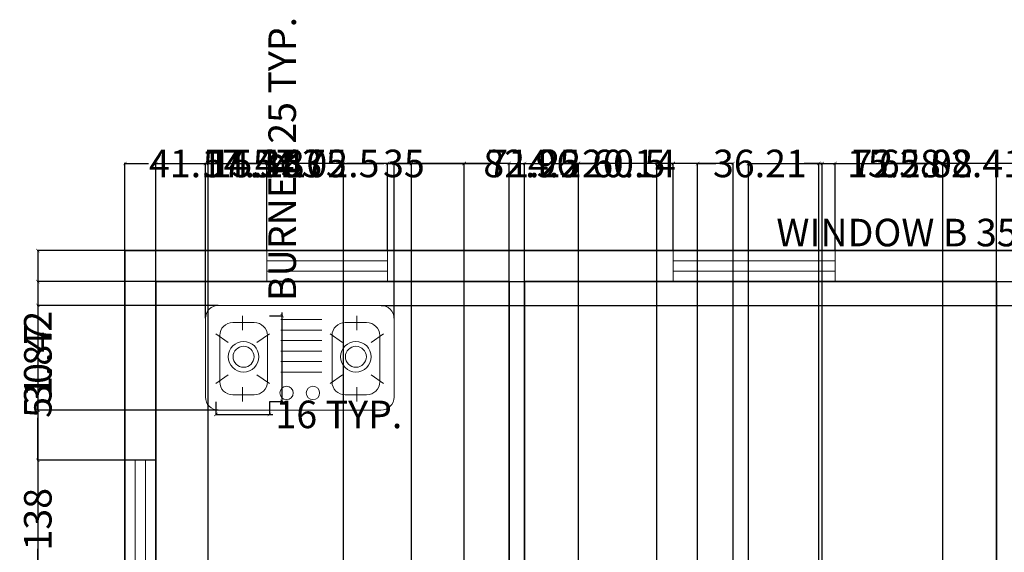
# Model space of a CAD drawing. Units: inches. Extents: x 878 to 1443, y 634 to 1188.
# Tile 3 of 5: x 878 to 1164, y 1033 to 1188. Entities that reach past the tile are written whole.
import ezdxf

# ---------------------------------------------------------------- set-up
doc = ezdxf.new("R2010")
doc.units = ezdxf.units.IN
doc.header["$MEASUREMENT"] = 0
doc.layers.add('A-ANNO-DIMS', color=2, linetype='Continuous', lineweight=18)
doc.layers.add('A-WALL', color=7, linetype='Continuous', lineweight=35)
doc.layers.add('A-GLAZ', color=152, linetype='Continuous', lineweight=18, true_color=0x2776bb)
doc.layers.add('Furniture', color=7, linetype='Continuous', lineweight=15, true_color=0xffffff)
doc.styles.get("Standard").update_dxf_attribs({"font": 'arial.ttf'})
doc.dimstyles.get("Standard").update_dxf_attribs({"dimtxt": 8, "dimasz": 1, "dimexe": 0.18, "dimexo": 0.0625, "dimgap": 0.09, "dimtad": 0, "dimdec": 4, "dimzin": 0, "dimdsep": 46, "dimlunit": 3, "dimtxsty": 'Standard', "dimblk": 'ARCHTICK', "dimcen": 0.09, "dimclrd": 6, "dimclre": 5, "dimclrt": 140, "dimadec": 0, "dimazin": 0, "dimtfac": 1, "dimtdec": 4, "dimtofl": 0, "dimtmove": 0, "dimatfit": 3, "dimfxl": 1, "dimtolj": 1, "dimtzin": 0, "dimarcsym": 0})

# ---------------------------------------------------------------- blocks, each defined once
blk = doc.blocks.new('WIN-47IN')
for p, q in [((9, 47), (0, 47)), ((0, 47), (0, 0)), ((3, 0), (3, 47)), ((6, 0), (6, 47)), ((9, 0), (9, 47)), ((0, 0), (9, 0))]:
    blk.add_line(p, q)
blk = doc.blocks.new('COOKTOP-BURNER')
for p, q in [((11.15, 22.96), (4.91, 22.96)), ((7.76, 24.89), (7.76, 20.74)), ((0, 19.64), (3.6, 17.15)), ((1.11, 19.15), (1.11, 5.74)), ((15.51, 19.64), (11.91, 17.15)), ((14.96, 5.74), (14.96, 19.15)), ((0, 5.25), (3.6, 7.74)), ((15.51, 5.25), (11.91, 7.74)), ((7.76, 0), (7.76, 4.15)), ((4.91, 1.94), (11.15, 1.94))]:
    blk.add_line(p, q)
for radius in [4.43, 3.05]:
    blk.add_circle((8.03, 13), radius)
for centre, start, end in [((4.91, 19.15), 90, 180), ((11.15, 19.15), 0, 90), ((4.91, 5.74), 180, 270), ((11.15, 5.74), 270, 0)]:
    blk.add_arc(centre, 3.8, start, end)
blk = doc.blocks.new('WIN-35IN')
for p, q in [((0, 35), (0, 0)), ((9, 35), (0, 35)), ((3, 0), (3, 35)), ((6, 0), (6, 35)), ((9, 0), (9, 35)), ((0, 0), (9, 0))]:
    blk.add_line(p, q)
blk = doc.blocks.new('_ArchTick')
at = {"color": 0, "linetype": 'ByBlock', "const_width": 0.15}
blk.add_lwpolyline([(-0.5, -0.5), (0.5, 0.5)], dxfattribs=at)
blk = doc.blocks.new('*D11')
at = {"layer": 'A-ANNO-DIMS', "color": 6, "lineweight": -2, "transparency": 16777216}
for p, q in [((1197.44, 1125.72), (1196.44, 1125.72)), ((1232.44, 1125.72), (1197.44, 1125.72))]:
    blk.add_line(p, q, dxfattribs=at)
at = {"layer": 'A-ANNO-DIMS', "color": 5, "lineweight": -2, "transparency": 16777216}
for p, q in [((1197.44, 1120.53), (1197.44, 1125.9)), ((1232.44, 1120.53), (1232.44, 1125.9))]:
    blk.add_line(p, q, dxfattribs=at)
at = {"layer": 'Defpoints', "color": 0, "lineweight": -2, "transparency": 16777216}
for p in [(1197.44, 1125.72), (1197.44, 1120.47), (1232.44, 1120.47)]:
    blk.add_point(p, dxfattribs=at)
at = {"layer": 'A-ANNO-DIMS', "color": 6, "lineweight": -2, "transparency": 16777216}
for p, rotation in [((1197.44, 1125.72), 179.9999999999992), ((1232.44, 1125.72), 359.9999999999992)]:
    blk.add_blockref('_ArchTick', p, dxfattribs=dict(at, rotation=rotation))
at = {"layer": 'A-ANNO-DIMS', "color": 140, "transparency": 16777216, "insert": (1145.37, 1125.72), "char_height": 8, "attachment_point": 5}
blk.add_mtext('\\A1;WINDOW B 35 TYP.', dxfattribs=at)
blk = doc.blocks.new('*D19')
at = {"layer": 'A-ANNO-DIMS', "color": 5, "lineweight": -2, "transparency": 16777216}
for p, q in [((950.87, 1101.54), (954.72, 1101.54)), ((950.87, 1076.65), (954.72, 1076.65))]:
    blk.add_line(p, q, dxfattribs=at)
at = {"layer": 'A-ANNO-DIMS', "color": 6, "lineweight": -2, "transparency": 16777216}
for p, q in [((954.54, 1101.54), (954.54, 1102.54)), ((954.54, 1076.65), (954.54, 1101.54))]:
    blk.add_line(p, q, dxfattribs=at)
at = {"layer": 'Defpoints', "color": 0, "lineweight": -2, "transparency": 16777216}
for p in [(950.81, 1101.54), (954.54, 1101.54), (950.81, 1076.65)]:
    blk.add_point(p, dxfattribs=at)
at = {"layer": 'A-ANNO-DIMS', "color": 6, "lineweight": -2, "transparency": 16777216}
for p, rotation in [((954.54, 1101.54), 90), ((954.54, 1076.65), 270)]:
    blk.add_blockref('_ArchTick', p, dxfattribs=dict(at, rotation=rotation))
at = {"layer": 'A-ANNO-DIMS', "color": 140, "transparency": 16777216, "insert": (954.54, 1147.08), "char_height": 8, "attachment_point": 5, "rotation": 90}
blk.add_mtext('\\A1;BURNER 25 TYP.', dxfattribs=at)
blk = doc.blocks.new('*D20')
at = {"layer": 'A-ANNO-DIMS', "color": 5, "lineweight": -2, "transparency": 16777216}
for p, q in [((935.3, 1076.59), (935.3, 1072.74)), ((950.81, 1076.59), (950.81, 1072.74))]:
    blk.add_line(p, q, dxfattribs=at)
at = {"layer": 'A-ANNO-DIMS', "color": 6, "lineweight": -2, "transparency": 16777216}
for p, q in [((935.3, 1072.92), (950.81, 1072.92)), ((950.81, 1072.92), (951.81, 1072.92))]:
    blk.add_line(p, q, dxfattribs=at)
at = {"layer": 'Defpoints', "color": 0, "lineweight": -2, "transparency": 16777216}
for p in [(935.3, 1076.65), (950.81, 1076.65), (950.81, 1072.92)]:
    blk.add_point(p, dxfattribs=at)
at = {"layer": 'A-ANNO-DIMS', "color": 6, "lineweight": -2, "transparency": 16777216, "rotation": 180}
blk.add_blockref('_ArchTick', (935.3, 1072.92), dxfattribs=at)
at = {"layer": 'A-ANNO-DIMS', "color": 6, "lineweight": -2, "transparency": 16777216}
blk.add_blockref('_ArchTick', (950.81, 1072.92), dxfattribs=at)
at = {"layer": 'A-ANNO-DIMS', "color": 140, "transparency": 16777216, "insert": (970.99, 1072.92), "char_height": 8, "attachment_point": 5}
blk.add_mtext('\\A1;16 TYP.', dxfattribs=at)
blk = doc.blocks.new('*D22')
at = {"layer": 'A-ANNO-DIMS', "color": 5, "lineweight": -2, "transparency": 16777216}
for p, q in [((908.84, 1120.47), (883.41, 1120.47)), ((908.84, 664.47), (883.41, 664.47))]:
    blk.add_line(p, q, dxfattribs=at)
at = {"layer": 'A-ANNO-DIMS', "color": 6, "lineweight": -2, "transparency": 16777216}
for p, q in [((883.59, 1120.47), (883.59, 901.56)), ((883.59, 664.47), (883.59, 883.38))]:
    blk.add_line(p, q, dxfattribs=at)
at = {"layer": 'Defpoints', "color": 0, "lineweight": -2, "transparency": 16777216}
for p in [(883.59, 1120.47), (908.9, 1120.47), (908.9, 664.47)]:
    blk.add_point(p, dxfattribs=at)
at = {"layer": 'A-ANNO-DIMS', "color": 6, "lineweight": -2, "transparency": 16777216}
for p, rotation in [((883.59, 1120.47), 90), ((883.59, 664.47), 270)]:
    blk.add_blockref('_ArchTick', p, dxfattribs=dict(at, rotation=rotation))
at = {"layer": 'A-ANNO-DIMS', "color": 140, "transparency": 16777216, "insert": (883.59, 892.47), "char_height": 8, "attachment_point": 5, "rotation": 90}
blk.add_mtext('\\A1;456', dxfattribs=at)
blk = doc.blocks.new('*D24')
at = {"layer": 'A-ANNO-DIMS', "color": 5, "lineweight": -2, "transparency": 16777216}
for p, q in [((908.9, 1120.53), (908.9, 1145.96)), ((950.07, 1120.53), (950.07, 1145.96))]:
    blk.add_line(p, q, dxfattribs=at)
at = {"layer": 'A-ANNO-DIMS', "color": 6, "lineweight": -2, "transparency": 16777216}
for p, q in [((908.9, 1145.78), (915.74, 1145.78)), ((950.07, 1145.78), (943.23, 1145.78))]:
    blk.add_line(p, q, dxfattribs=at)
at = {"layer": 'Defpoints', "color": 0, "lineweight": -2, "transparency": 16777216}
for p in [(950.07, 1145.78), (908.9, 1120.47), (950.07, 1120.47)]:
    blk.add_point(p, dxfattribs=at)
at = {"layer": 'A-ANNO-DIMS', "color": 6, "lineweight": -2, "transparency": 16777216, "rotation": 180}
blk.add_blockref('_ArchTick', (908.9, 1145.78), dxfattribs=at)
at = {"layer": 'A-ANNO-DIMS', "color": 6, "lineweight": -2, "transparency": 16777216}
blk.add_blockref('_ArchTick', (950.07, 1145.78), dxfattribs=at)
at = {"layer": 'A-ANNO-DIMS', "color": 140, "transparency": 16777216, "insert": (929.49, 1145.78), "char_height": 8, "attachment_point": 5}
blk.add_mtext('\\A1;41.17', dxfattribs=at)
blk = doc.blocks.new('*D25')
at = {"layer": 'A-ANNO-DIMS', "color": 5, "lineweight": -2, "transparency": 16777216}
for p, q in [((985.07, 1120.53), (985.07, 1145.96)), ((1068.03, 1120.53), (1068.03, 1145.96))]:
    blk.add_line(p, q, dxfattribs=at)
at = {"layer": 'A-ANNO-DIMS', "color": 6, "lineweight": -2, "transparency": 16777216}
for p, q in [((985.07, 1145.78), (1012.96, 1145.78)), ((1068.03, 1145.78), (1040.14, 1145.78))]:
    blk.add_line(p, q, dxfattribs=at)
at = {"layer": 'Defpoints', "color": 0, "lineweight": -2, "transparency": 16777216}
for p in [(1068.03, 1145.78), (985.07, 1120.47), (1068.03, 1120.47)]:
    blk.add_point(p, dxfattribs=at)
at = {"layer": 'A-ANNO-DIMS', "color": 6, "lineweight": -2, "transparency": 16777216, "rotation": 180}
blk.add_blockref('_ArchTick', (985.07, 1145.78), dxfattribs=at)
at = {"layer": 'A-ANNO-DIMS', "color": 6, "lineweight": -2, "transparency": 16777216}
blk.add_blockref('_ArchTick', (1068.03, 1145.78), dxfattribs=at)
at = {"layer": 'A-ANNO-DIMS', "color": 140, "transparency": 16777216, "insert": (1026.55, 1145.78), "char_height": 8, "attachment_point": 5}
blk.add_mtext('\\A1;82.96', dxfattribs=at)
blk = doc.blocks.new('*D26')
at = {"layer": 'A-ANNO-DIMS', "color": 5, "lineweight": -2, "transparency": 16777216}
for p, q in [((1115.03, 1120.53), (1115.03, 1145.96)), ((1197.44, 1120.53), (1197.44, 1145.96))]:
    blk.add_line(p, q, dxfattribs=at)
at = {"layer": 'A-ANNO-DIMS', "color": 6, "lineweight": -2, "transparency": 16777216}
for p, q in [((1115.03, 1145.78), (1143.42, 1145.78)), ((1197.44, 1145.78), (1169.06, 1145.78))]:
    blk.add_line(p, q, dxfattribs=at)
at = {"layer": 'Defpoints', "color": 0, "lineweight": -2, "transparency": 16777216}
for p in [(1197.44, 1145.78), (1115.03, 1120.47), (1197.44, 1120.47)]:
    blk.add_point(p, dxfattribs=at)
at = {"layer": 'A-ANNO-DIMS', "color": 6, "lineweight": -2, "transparency": 16777216, "rotation": 180}
blk.add_blockref('_ArchTick', (1115.03, 1145.78), dxfattribs=at)
at = {"layer": 'A-ANNO-DIMS', "color": 6, "lineweight": -2, "transparency": 16777216}
blk.add_blockref('_ArchTick', (1197.44, 1145.78), dxfattribs=at)
at = {"layer": 'A-ANNO-DIMS', "color": 140, "transparency": 16777216, "insert": (1156.24, 1145.78), "char_height": 8, "attachment_point": 5}
blk.add_mtext('\\A1;82.41', dxfattribs=at)
blk = doc.blocks.new('*D29')
at = {"layer": 'A-ANNO-DIMS', "color": 5, "lineweight": -2, "transparency": 16777216}
for p, q in [((917.84, 1111.47), (883.41, 1111.47)), ((917.84, 1059.6), (883.41, 1059.6))]:
    blk.add_line(p, q, dxfattribs=at)
at = {"layer": 'A-ANNO-DIMS', "color": 6, "lineweight": -2, "transparency": 16777216}
for p, q in [((883.59, 1111.47), (883.59, 1099.12)), ((883.59, 1059.6), (883.59, 1071.95))]:
    blk.add_line(p, q, dxfattribs=at)
at = {"layer": 'Defpoints', "color": 0, "lineweight": -2, "transparency": 16777216}
for p in [(917.9, 1111.47), (883.59, 1059.6), (917.9, 1059.6)]:
    blk.add_point(p, dxfattribs=at)
at = {"layer": 'A-ANNO-DIMS', "color": 6, "lineweight": -2, "transparency": 16777216}
for p, rotation in [((883.59, 1111.47), 90), ((883.59, 1059.6), 270)]:
    blk.add_blockref('_ArchTick', p, dxfattribs=dict(at, rotation=rotation))
at = {"layer": 'A-ANNO-DIMS', "color": 140, "transparency": 16777216, "insert": (883.59, 1085.53), "char_height": 8, "attachment_point": 5, "rotation": 90}
blk.add_mtext('\\A1;51.87', dxfattribs=at)
blk = doc.blocks.new('*D33')
at = {"layer": 'A-ANNO-DIMS', "color": 5, "lineweight": -2, "transparency": 16777216}
for p, q in [((917.9, 760.53), (917.9, 1145.96)), ((1020.4, 760.53), (1020.4, 1145.96))]:
    blk.add_line(p, q, dxfattribs=at)
at = {"layer": 'A-ANNO-DIMS', "color": 6, "lineweight": -2, "transparency": 16777216}
for p, q in [((917.9, 1145.78), (955.91, 1145.78)), ((1020.4, 1145.78), (982.39, 1145.78))]:
    blk.add_line(p, q, dxfattribs=at)
at = {"layer": 'Defpoints', "color": 0, "lineweight": -2, "transparency": 16777216}
for p in [(1020.4, 1145.78), (917.9, 760.47), (1020.4, 760.47)]:
    blk.add_point(p, dxfattribs=at)
at = {"layer": 'A-ANNO-DIMS', "color": 6, "lineweight": -2, "transparency": 16777216, "rotation": 180}
blk.add_blockref('_ArchTick', (917.9, 1145.78), dxfattribs=at)
at = {"layer": 'A-ANNO-DIMS', "color": 6, "lineweight": -2, "transparency": 16777216}
blk.add_blockref('_ArchTick', (1020.4, 1145.78), dxfattribs=at)
at = {"layer": 'A-ANNO-DIMS', "color": 140, "transparency": 16777216, "insert": (969.15, 1145.78), "char_height": 8, "attachment_point": 5}
blk.add_mtext('\\A1;102.5', dxfattribs=at)
blk = doc.blocks.new('*D34')
at = {"layer": 'A-ANNO-DIMS', "color": 5, "lineweight": -2, "transparency": 16777216}
for p, q in [((1024.9, 1111.41), (1024.9, 638.98)), ((1161.9, 1111.41), (1161.9, 638.98))]:
    blk.add_line(p, q, dxfattribs=at)
at = {"layer": 'A-ANNO-DIMS', "color": 6, "lineweight": -2, "transparency": 16777216}
for p, q in [((1024.9, 639.16), (1084.85, 639.16)), ((1161.9, 639.16), (1101.95, 639.16))]:
    blk.add_line(p, q, dxfattribs=at)
at = {"layer": 'Defpoints', "color": 0, "lineweight": -2, "transparency": 16777216}
for p in [(1024.9, 1111.47), (1161.9, 1111.47), (1161.9, 639.16)]:
    blk.add_point(p, dxfattribs=at)
at = {"layer": 'A-ANNO-DIMS', "color": 6, "lineweight": -2, "transparency": 16777216, "rotation": 180}
blk.add_blockref('_ArchTick', (1024.9, 639.16), dxfattribs=at)
at = {"layer": 'A-ANNO-DIMS', "color": 6, "lineweight": -2, "transparency": 16777216}
blk.add_blockref('_ArchTick', (1161.9, 639.16), dxfattribs=at)
at = {"layer": 'A-ANNO-DIMS', "color": 140, "transparency": 16777216, "insert": (1093.4, 639.16), "char_height": 8, "attachment_point": 5}
blk.add_mtext('\\A1;137', dxfattribs=at)
blk = doc.blocks.new('*D36')
at = {"layer": 'A-ANNO-DIMS', "color": 5, "lineweight": -2, "transparency": 16777216}
for p, q in [((1020.34, 1111.47), (883.41, 1111.47)), ((1020.34, 973.47), (883.41, 973.47))]:
    blk.add_line(p, q, dxfattribs=at)
at = {"layer": 'A-ANNO-DIMS', "color": 6, "lineweight": -2, "transparency": 16777216}
for p, q in [((883.59, 1111.47), (883.59, 1051.03)), ((883.59, 973.47), (883.59, 1033.91))]:
    blk.add_line(p, q, dxfattribs=at)
at = {"layer": 'Defpoints', "color": 0, "lineweight": -2, "transparency": 16777216}
for p in [(1020.4, 1111.47), (883.59, 973.47), (1020.4, 973.47)]:
    blk.add_point(p, dxfattribs=at)
at = {"layer": 'A-ANNO-DIMS', "color": 6, "lineweight": -2, "transparency": 16777216}
for p, rotation in [((883.59, 1111.47), 90), ((883.59, 973.47), 270)]:
    blk.add_blockref('_ArchTick', p, dxfattribs=dict(at, rotation=rotation))
at = {"layer": 'A-ANNO-DIMS', "color": 140, "transparency": 16777216, "insert": (883.59, 1042.47), "char_height": 8, "attachment_point": 5, "rotation": 90}
blk.add_mtext('\\A1;138', dxfattribs=at)
blk = doc.blocks.new('*D39')
at = {"layer": 'A-ANNO-DIMS', "color": 5, "lineweight": -2, "transparency": 16777216}
for p, q in [((1024.9, 880.53), (1024.9, 1145.96)), ((1085.4, 880.53), (1085.4, 1145.96))]:
    blk.add_line(p, q, dxfattribs=at)
at = {"layer": 'A-ANNO-DIMS', "color": 6, "lineweight": -2, "transparency": 16777216}
for p, q in [((1024.9, 1145.78), (1044.62, 1145.78)), ((1085.4, 1145.78), (1065.68, 1145.78))]:
    blk.add_line(p, q, dxfattribs=at)
at = {"layer": 'Defpoints', "color": 0, "lineweight": -2, "transparency": 16777216}
for p in [(1085.4, 1145.78), (1024.9, 880.47), (1085.4, 880.47)]:
    blk.add_point(p, dxfattribs=at)
at = {"layer": 'A-ANNO-DIMS', "color": 6, "lineweight": -2, "transparency": 16777216, "rotation": 180}
blk.add_blockref('_ArchTick', (1024.9, 1145.78), dxfattribs=at)
at = {"layer": 'A-ANNO-DIMS', "color": 6, "lineweight": -2, "transparency": 16777216}
blk.add_blockref('_ArchTick', (1085.4, 1145.78), dxfattribs=at)
at = {"layer": 'A-ANNO-DIMS', "color": 140, "transparency": 16777216, "insert": (1055.15, 1145.78), "char_height": 8, "attachment_point": 5}
blk.add_mtext('\\A1;60.5', dxfattribs=at)
blk = doc.blocks.new('*D40')
at = {"layer": 'A-ANNO-DIMS', "color": 5, "lineweight": -2, "transparency": 16777216}
for p, q in [((1089.9, 880.53), (1089.9, 1145.96)), ((1161.9, 880.53), (1161.9, 1145.96))]:
    blk.add_line(p, q, dxfattribs=at)
at = {"layer": 'A-ANNO-DIMS', "color": 6, "lineweight": -2, "transparency": 16777216}
for p, q in [((1089.9, 1145.78), (1120.15, 1145.78)), ((1161.9, 1145.78), (1131.64, 1145.78))]:
    blk.add_line(p, q, dxfattribs=at)
at = {"layer": 'Defpoints', "color": 0, "lineweight": -2, "transparency": 16777216}
for p in [(1161.9, 1145.78), (1089.9, 880.47), (1161.9, 880.47)]:
    blk.add_point(p, dxfattribs=at)
at = {"layer": 'A-ANNO-DIMS', "color": 6, "lineweight": -2, "transparency": 16777216, "rotation": 180}
blk.add_blockref('_ArchTick', (1089.9, 1145.78), dxfattribs=at)
at = {"layer": 'A-ANNO-DIMS', "color": 6, "lineweight": -2, "transparency": 16777216}
blk.add_blockref('_ArchTick', (1161.9, 1145.78), dxfattribs=at)
at = {"layer": 'A-ANNO-DIMS', "color": 140, "transparency": 16777216, "insert": (1125.9, 1145.78), "char_height": 8, "attachment_point": 5}
blk.add_mtext('\\A1;72', dxfattribs=at)
blk = doc.blocks.new('*D44')
at = {"layer": 'A-ANNO-DIMS', "color": 5, "lineweight": -2, "transparency": 16777216}
for p, q in [((917.9, 751.53), (917.9, 1145.96)), ((933.09, 751.53), (933.09, 1145.96))]:
    blk.add_line(p, q, dxfattribs=at)
at = {"layer": 'A-ANNO-DIMS', "color": 6, "lineweight": -2, "transparency": 16777216}
for p, q in [((917.9, 1145.78), (933.09, 1145.78)), ((933.09, 1145.78), (934.09, 1145.78))]:
    blk.add_line(p, q, dxfattribs=at)
at = {"layer": 'Defpoints', "color": 0, "lineweight": -2, "transparency": 16777216}
for p in [(933.09, 1145.78), (917.9, 751.47), (933.09, 751.47)]:
    blk.add_point(p, dxfattribs=at)
at = {"layer": 'A-ANNO-DIMS', "color": 6, "lineweight": -2, "transparency": 16777216, "rotation": 180}
blk.add_blockref('_ArchTick', (917.9, 1145.78), dxfattribs=at)
at = {"layer": 'A-ANNO-DIMS', "color": 6, "lineweight": -2, "transparency": 16777216}
blk.add_blockref('_ArchTick', (933.09, 1145.78), dxfattribs=at)
at = {"layer": 'A-ANNO-DIMS', "color": 140, "transparency": 16777216, "insert": (950.4, 1145.78), "char_height": 8, "attachment_point": 5}
blk.add_mtext('\\A1;15.187', dxfattribs=at)
blk = doc.blocks.new('*D45')
at = {"layer": 'A-ANNO-DIMS', "color": 5, "lineweight": -2, "transparency": 16777216}
for p, q in [((992.09, 751.53), (992.09, 1145.96)), ((1063.3, 751.53), (1063.3, 1145.96))]:
    blk.add_line(p, q, dxfattribs=at)
at = {"layer": 'A-ANNO-DIMS', "color": 6, "lineweight": -2, "transparency": 16777216}
for p, q in [((992.09, 1145.78), (1014.18, 1145.78)), ((1063.3, 1145.78), (1041.21, 1145.78))]:
    blk.add_line(p, q, dxfattribs=at)
at = {"layer": 'Defpoints', "color": 0, "lineweight": -2, "transparency": 16777216}
for p in [(1063.3, 1145.78), (992.09, 751.47), (1063.3, 751.47)]:
    blk.add_point(p, dxfattribs=at)
at = {"layer": 'A-ANNO-DIMS', "color": 6, "lineweight": -2, "transparency": 16777216, "rotation": 180}
blk.add_blockref('_ArchTick', (992.09, 1145.78), dxfattribs=at)
at = {"layer": 'A-ANNO-DIMS', "color": 6, "lineweight": -2, "transparency": 16777216}
blk.add_blockref('_ArchTick', (1063.3, 1145.78), dxfattribs=at)
at = {"layer": 'A-ANNO-DIMS', "color": 140, "transparency": 16777216, "insert": (1027.69, 1145.78), "char_height": 8, "attachment_point": 5}
blk.add_mtext('\\A1;71.22', dxfattribs=at)
blk = doc.blocks.new('*D46')
at = {"layer": 'A-ANNO-DIMS', "color": 5, "lineweight": -2, "transparency": 16777216}
for p, q in [((1110.3, 751.53), (1110.3, 1145.96)), ((1172.39, 751.53), (1172.39, 1145.96))]:
    blk.add_line(p, q, dxfattribs=at)
at = {"layer": 'A-ANNO-DIMS', "color": 6, "lineweight": -2, "transparency": 16777216}
for p, q in [((1110.3, 1145.78), (1127.73, 1145.78)), ((1172.39, 1145.78), (1154.96, 1145.78))]:
    blk.add_line(p, q, dxfattribs=at)
at = {"layer": 'Defpoints', "color": 0, "lineweight": -2, "transparency": 16777216}
for p in [(1172.39, 1145.78), (1110.3, 751.47), (1172.39, 751.47)]:
    blk.add_point(p, dxfattribs=at)
at = {"layer": 'A-ANNO-DIMS', "color": 6, "lineweight": -2, "transparency": 16777216, "rotation": 180}
blk.add_blockref('_ArchTick', (1110.3, 1145.78), dxfattribs=at)
at = {"layer": 'A-ANNO-DIMS', "color": 6, "lineweight": -2, "transparency": 16777216}
blk.add_blockref('_ArchTick', (1172.39, 1145.78), dxfattribs=at)
at = {"layer": 'A-ANNO-DIMS', "color": 140, "transparency": 16777216, "insert": (1141.35, 1145.78), "char_height": 8, "attachment_point": 5}
blk.add_mtext('\\A1;62.08', dxfattribs=at)
blk = doc.blocks.new('*D49')
at = {"layer": 'A-ANNO-DIMS', "color": 5, "lineweight": -2, "transparency": 16777216}
for p, q in [((917.9, 973.53), (917.9, 1145.96)), ((972.37, 973.53), (972.37, 1145.96))]:
    blk.add_line(p, q, dxfattribs=at)
at = {"layer": 'A-ANNO-DIMS', "color": 6, "lineweight": -2, "transparency": 16777216}
for p, q in [((917.9, 1145.78), (931.54, 1145.78)), ((972.37, 1145.78), (958.72, 1145.78))]:
    blk.add_line(p, q, dxfattribs=at)
at = {"layer": 'Defpoints', "color": 0, "lineweight": -2, "transparency": 16777216}
for p in [(972.37, 1145.78), (917.9, 973.47), (972.37, 973.47)]:
    blk.add_point(p, dxfattribs=at)
at = {"layer": 'A-ANNO-DIMS', "color": 6, "lineweight": -2, "transparency": 16777216, "rotation": 180}
blk.add_blockref('_ArchTick', (917.9, 1145.78), dxfattribs=at)
at = {"layer": 'A-ANNO-DIMS', "color": 6, "lineweight": -2, "transparency": 16777216}
blk.add_blockref('_ArchTick', (972.37, 1145.78), dxfattribs=at)
at = {"layer": 'A-ANNO-DIMS', "color": 140, "transparency": 16777216, "insert": (945.13, 1145.78), "char_height": 8, "attachment_point": 5}
blk.add_mtext('\\A1;54.47', dxfattribs=at)
blk = doc.blocks.new('*D50')
at = {"layer": 'A-ANNO-DIMS', "color": 5, "lineweight": -2, "transparency": 16777216}
for p, q in [((972.37, 973.53), (972.37, 1145.96)), ((1007.37, 973.53), (1007.37, 1145.96))]:
    blk.add_line(p, q, dxfattribs=at)
at = {"layer": 'A-ANNO-DIMS', "color": 6, "lineweight": -2, "transparency": 16777216}
for p, q in [((972.37, 1145.78), (984.02, 1145.78)), ((1007.37, 1145.78), (995.71, 1145.78))]:
    blk.add_line(p, q, dxfattribs=at)
at = {"layer": 'Defpoints', "color": 0, "lineweight": -2, "transparency": 16777216}
for p in [(1007.37, 1145.78), (972.37, 973.47), (1007.37, 973.47)]:
    blk.add_point(p, dxfattribs=at)
at = {"layer": 'A-ANNO-DIMS', "color": 6, "lineweight": -2, "transparency": 16777216, "rotation": 180}
blk.add_blockref('_ArchTick', (972.37, 1145.78), dxfattribs=at)
at = {"layer": 'A-ANNO-DIMS', "color": 6, "lineweight": -2, "transparency": 16777216}
blk.add_blockref('_ArchTick', (1007.37, 1145.78), dxfattribs=at)
at = {"layer": 'A-ANNO-DIMS', "color": 140, "transparency": 16777216, "insert": (989.87, 1145.78), "char_height": 8, "attachment_point": 5}
blk.add_mtext('\\A1;35', dxfattribs=at)
blk = doc.blocks.new('*D52')
at = {"layer": 'A-ANNO-DIMS', "color": 6, "lineweight": -2, "transparency": 16777216}
for p, q in [((1146.32, 1145.78), (1145.32, 1145.78)), ((1161.9, 1145.78), (1146.32, 1145.78))]:
    blk.add_line(p, q, dxfattribs=at)
at = {"layer": 'A-ANNO-DIMS', "color": 5, "lineweight": -2, "transparency": 16777216}
for p, q in [((1146.32, 973.53), (1146.32, 1145.96)), ((1161.9, 973.53), (1161.9, 1145.96))]:
    blk.add_line(p, q, dxfattribs=at)
at = {"layer": 'Defpoints', "color": 0, "lineweight": -2, "transparency": 16777216}
for p in [(1146.32, 1145.78), (1146.32, 973.47), (1161.9, 973.47)]:
    blk.add_point(p, dxfattribs=at)
at = {"layer": 'A-ANNO-DIMS', "color": 6, "lineweight": -2, "transparency": 16777216, "rotation": 180}
blk.add_blockref('_ArchTick', (1146.32, 1145.78), dxfattribs=at)
at = {"layer": 'A-ANNO-DIMS', "color": 6, "lineweight": -2, "transparency": 16777216}
blk.add_blockref('_ArchTick', (1161.9, 1145.78), dxfattribs=at)
at = {"layer": 'A-ANNO-DIMS', "color": 140, "transparency": 16777216, "insert": (1132.1, 1145.78), "char_height": 8, "attachment_point": 5}
blk.add_mtext('\\A1;15.58', dxfattribs=at)
blk = doc.blocks.new('*D53')
at = {"layer": 'A-ANNO-DIMS', "color": 5, "lineweight": -2, "transparency": 16777216}
for p, q in [((1075.11, 1016.03), (1075.11, 1145.96)), ((1111.32, 1004.03), (1111.32, 1145.96))]:
    blk.add_line(p, q, dxfattribs=at)
at = {"layer": 'A-ANNO-DIMS', "color": 6, "lineweight": -2, "transparency": 16777216}
for p, q in [((1075.11, 1145.78), (1080.4, 1145.78)), ((1111.32, 1145.78), (1106.03, 1145.78))]:
    blk.add_line(p, q, dxfattribs=at)
at = {"layer": 'Defpoints', "color": 0, "lineweight": -2, "transparency": 16777216}
for p in [(1111.32, 1145.78), (1075.11, 1015.97), (1111.32, 1003.97)]:
    blk.add_point(p, dxfattribs=at)
at = {"layer": 'A-ANNO-DIMS', "color": 6, "lineweight": -2, "transparency": 16777216, "rotation": 180}
blk.add_blockref('_ArchTick', (1075.11, 1145.78), dxfattribs=at)
at = {"layer": 'A-ANNO-DIMS', "color": 6, "lineweight": -2, "transparency": 16777216}
blk.add_blockref('_ArchTick', (1111.32, 1145.78), dxfattribs=at)
at = {"layer": 'A-ANNO-DIMS', "color": 140, "transparency": 16777216, "insert": (1093.21, 1145.78), "char_height": 8, "attachment_point": 5}
blk.add_mtext('\\A1;36.21', dxfattribs=at)
blk = doc.blocks.new('*D56')
at = {"layer": 'A-ANNO-DIMS', "color": 5, "lineweight": -2, "transparency": 16777216}
for p, q in [((1020.4, 936.63), (1020.4, 1145.96)), ((1040.54, 936.63), (1040.54, 1145.96))]:
    blk.add_line(p, q, dxfattribs=at)
at = {"layer": 'A-ANNO-DIMS', "color": 6, "lineweight": -2, "transparency": 16777216}
for p, q in [((1020.4, 1145.78), (1040.54, 1145.78)), ((1040.54, 1145.78), (1041.54, 1145.78))]:
    blk.add_line(p, q, dxfattribs=at)
at = {"layer": 'Defpoints', "color": 0, "lineweight": -2, "transparency": 16777216}
for p in [(1040.54, 1145.78), (1020.4, 936.57), (1040.54, 936.57)]:
    blk.add_point(p, dxfattribs=at)
at = {"layer": 'A-ANNO-DIMS', "color": 6, "lineweight": -2, "transparency": 16777216, "rotation": 180}
blk.add_blockref('_ArchTick', (1020.4, 1145.78), dxfattribs=at)
at = {"layer": 'A-ANNO-DIMS', "color": 6, "lineweight": -2, "transparency": 16777216}
blk.add_blockref('_ArchTick', (1040.54, 1145.78), dxfattribs=at)
at = {"layer": 'A-ANNO-DIMS', "color": 140, "transparency": 16777216, "insert": (1055.18, 1145.78), "char_height": 8, "attachment_point": 5}
blk.add_mtext('\\A1;20.14', dxfattribs=at)
blk = doc.blocks.new('*D63')
at = {"layer": 'A-ANNO-DIMS', "color": 5, "lineweight": -2, "transparency": 16777216}
for p, q in [((1020.4, 851.67), (1020.4, 1145.96)), ((1024.9, 851.67), (1024.9, 1145.96))]:
    blk.add_line(p, q, dxfattribs=at)
at = {"layer": 'A-ANNO-DIMS', "color": 6, "lineweight": -2, "transparency": 16777216}
for p, q in [((1020.4, 1145.78), (1024.9, 1145.78)), ((1024.9, 1145.78), (1025.9, 1145.78))]:
    blk.add_line(p, q, dxfattribs=at)
at = {"layer": 'Defpoints', "color": 0, "lineweight": -2, "transparency": 16777216}
for p in [(1024.9, 1145.78), (1020.4, 851.61), (1024.9, 851.61)]:
    blk.add_point(p, dxfattribs=at)
at = {"layer": 'A-ANNO-DIMS', "color": 6, "lineweight": -2, "transparency": 16777216, "rotation": 180}
blk.add_blockref('_ArchTick', (1020.4, 1145.78), dxfattribs=at)
at = {"layer": 'A-ANNO-DIMS', "color": 6, "lineweight": -2, "transparency": 16777216}
blk.add_blockref('_ArchTick', (1024.9, 1145.78), dxfattribs=at)
at = {"layer": 'A-ANNO-DIMS', "color": 140, "transparency": 16777216, "insert": (1033.46, 1145.78), "char_height": 8, "attachment_point": 5}
blk.add_mtext('\\A1;4.5', dxfattribs=at)
blk = doc.blocks.new('*D64')
at = {"layer": 'A-ANNO-DIMS', "color": 5, "lineweight": -2, "transparency": 16777216}
for p, q in [((932.25, 1100.84), (932.25, 1145.96)), ((987.01, 1100.84), (987.01, 1145.96))]:
    blk.add_line(p, q, dxfattribs=at)
at = {"layer": 'A-ANNO-DIMS', "color": 6, "lineweight": -2, "transparency": 16777216}
for p, q in [((932.25, 1145.78), (946.01, 1145.78)), ((987.01, 1145.78), (973.25, 1145.78))]:
    blk.add_line(p, q, dxfattribs=at)
at = {"layer": 'Defpoints', "color": 0, "lineweight": -2, "transparency": 16777216}
for p in [(987.01, 1145.78), (932.25, 1100.78), (987.01, 1100.78)]:
    blk.add_point(p, dxfattribs=at)
at = {"layer": 'A-ANNO-DIMS', "color": 6, "lineweight": -2, "transparency": 16777216, "rotation": 180}
blk.add_blockref('_ArchTick', (932.25, 1145.78), dxfattribs=at)
at = {"layer": 'A-ANNO-DIMS', "color": 6, "lineweight": -2, "transparency": 16777216}
blk.add_blockref('_ArchTick', (987.01, 1145.78), dxfattribs=at)
at = {"layer": 'A-ANNO-DIMS', "color": 140, "transparency": 16777216, "insert": (959.63, 1145.78), "char_height": 8, "attachment_point": 5}
blk.add_mtext('\\A1;54.75', dxfattribs=at)
blk = doc.blocks.new('*D65')
at = {"layer": 'A-ANNO-DIMS', "color": 5, "lineweight": -2, "transparency": 16777216}
for p, q in [((935.99, 1104.58), (883.41, 1104.58)), ((935.99, 1074.16), (883.41, 1074.16))]:
    blk.add_line(p, q, dxfattribs=at)
at = {"layer": 'A-ANNO-DIMS', "color": 6, "lineweight": -2, "transparency": 16777216}
for p, q in [((883.59, 1104.58), (883.59, 1102.92)), ((883.59, 1074.16), (883.59, 1075.83))]:
    blk.add_line(p, q, dxfattribs=at)
at = {"layer": 'Defpoints', "color": 0, "lineweight": -2, "transparency": 16777216}
for p in [(883.59, 1104.58), (936.05, 1104.58), (936.05, 1074.16)]:
    blk.add_point(p, dxfattribs=at)
at = {"layer": 'A-ANNO-DIMS', "color": 6, "lineweight": -2, "transparency": 16777216}
for p, rotation in [((883.59, 1104.58), 90), ((883.59, 1074.16), 270)]:
    blk.add_blockref('_ArchTick', p, dxfattribs=dict(at, rotation=rotation))
at = {"layer": 'A-ANNO-DIMS', "color": 140, "transparency": 16777216, "insert": (883.59, 1089.37), "char_height": 8, "attachment_point": 5, "rotation": 90}
blk.add_mtext('\\A1;30.42', dxfattribs=at)
blk = doc.blocks.new('*D66')
at = {"layer": 'A-ANNO-DIMS', "color": 5, "lineweight": -2, "transparency": 16777216}
for p, q in [((917.9, 1111.53), (917.9, 1145.96)), ((932.25, 1100.84), (932.25, 1145.96))]:
    blk.add_line(p, q, dxfattribs=at)
at = {"layer": 'A-ANNO-DIMS', "color": 6, "lineweight": -2, "transparency": 16777216}
for p, q in [((917.9, 1145.78), (932.25, 1145.78)), ((932.25, 1145.78), (933.25, 1145.78))]:
    blk.add_line(p, q, dxfattribs=at)
at = {"layer": 'Defpoints', "color": 0, "lineweight": -2, "transparency": 16777216}
for p in [(932.25, 1145.78), (917.9, 1111.47), (932.25, 1100.78)]:
    blk.add_point(p, dxfattribs=at)
at = {"layer": 'A-ANNO-DIMS', "color": 6, "lineweight": -2, "transparency": 16777216, "rotation": 180}
blk.add_blockref('_ArchTick', (917.9, 1145.78), dxfattribs=at)
at = {"layer": 'A-ANNO-DIMS', "color": 6, "lineweight": -2, "transparency": 16777216}
blk.add_blockref('_ArchTick', (932.25, 1145.78), dxfattribs=at)
at = {"layer": 'A-ANNO-DIMS', "color": 140, "transparency": 16777216, "insert": (949.57, 1145.78), "char_height": 8, "attachment_point": 5}
blk.add_mtext('\\A1;14.353', dxfattribs=at)
blk = doc.blocks.new('*D67')
at = {"layer": 'A-ANNO-DIMS', "color": 5, "lineweight": -2, "transparency": 16777216}
for p, q in [((985.14, 1111.47), (1438.39, 1111.47)), ((983.27, 1104.58), (1438.39, 1104.58))]:
    blk.add_line(p, q, dxfattribs=at)
at = {"layer": 'A-ANNO-DIMS', "color": 6, "lineweight": -2, "transparency": 16777216}
for p, q in [((1438.21, 1111.47), (1438.21, 1104.58)), ((1438.21, 1104.58), (1438.21, 1103.58))]:
    blk.add_line(p, q, dxfattribs=at)
at = {"layer": 'Defpoints', "color": 0, "lineweight": -2, "transparency": 16777216}
for p in [(985.07, 1111.47), (983.2, 1104.58), (1438.21, 1104.58)]:
    blk.add_point(p, dxfattribs=at)
at = {"layer": 'A-ANNO-DIMS', "color": 6, "lineweight": -2, "transparency": 16777216}
for p, rotation in [((1438.21, 1111.47), 90), ((1438.21, 1104.58), 270)]:
    blk.add_blockref('_ArchTick', p, dxfattribs=dict(at, rotation=rotation))
at = {"layer": 'A-ANNO-DIMS', "color": 140, "transparency": 16777216, "insert": (1438.21, 1089.96), "char_height": 8, "attachment_point": 5, "rotation": 90}
blk.add_mtext('\\A1;6.889', dxfattribs=at)

msp = doc.modelspace()

# ---------------------------------------------------------------- linework, layer by layer
at = {"layer": 'A-WALL'}
for p, q in [((908.8987, 1120.4702), (1412.8987, 1120.4702)), ((908.8987, 664.4702), (908.8987, 1120.4702)), ((917.8987, 1111.4702), (1020.3987, 1111.4702)), ((917.8987, 973.4702), (917.8987, 1111.4702)), ((1020.3987, 1111.4702), (1020.3987, 973.4702)), ((1024.8987, 1111.4702), (1024.8987, 973.4702)), ((1024.8987, 1111.4702), (1161.8987, 1111.4702)), ((1161.8987, 1111.4702), (1161.8987, 973.4702))]:
    msp.add_line(p, q, dxfattribs=at)
at = {"layer": 'Furniture'}
for p, q in [((936.0536, 1104.5815), (983.2032, 1104.5815)), ((932.2512, 1077.9648), (932.2512, 1100.7791)), ((954.1323, 1100.437), (966.0422, 1100.437)), ((987.0056, 1100.7791), (987.0056, 1077.9648)), ((954.1323, 1097.395), (966.0422, 1097.395)), ((954.1323, 1094.3531), (966.0422, 1094.3531)), ((954.1323, 1091.3112), (966.0422, 1091.3112)), ((954.1323, 1088.2693), (966.0422, 1088.2693)), ((954.1323, 1085.2274), (966.0422, 1085.2274)), ((983.2032, 1074.1624), (936.0536, 1074.1624))]:
    msp.add_line(p, q, dxfattribs=at)
for centre in [(955.7941, 1079.1407), (963.4627, 1079.1407)]:
    msp.add_circle(centre, 1.9388, dxfattribs=at)
for centre, start, end in [((936.0536, 1100.7791), 90, 180), ((983.2032, 1100.7791), 0, 90), ((936.0536, 1077.9648), 180, 270), ((983.2032, 1077.9648), 270, 0)]:
    msp.add_arc(centre, 3.8024, start, end, dxfattribs=at)

# ---------------------------------------------------------------- block references
at = {"layer": 'A-GLAZ'}
for name, p, rotation in [('WIN-35IN', (985.0726, 1111.4702), 89.9999999999992), ('WIN-47IN', (1068.0314, 1120.4702), 269.9999999999993)]:
    msp.add_blockref(name, p, dxfattribs=dict(at, rotation=rotation))
msp.add_blockref('WIN-47IN', (908.8987, 1012.5982), dxfattribs=at)
at = {"layer": 'Furniture'}
msp.add_blockref('COOKTOP-BURNER', (935.2979, 1076.6516), dxfattribs=at)
at = {"layer": 'Furniture', "extrusion": (0, 0, -1), "zscale": -1}
msp.add_blockref('COOKTOP-BURNER', (-983.9589, 1076.6516), dxfattribs=at)

# ---------------------------------------------------------------- dimensions: what is measured, and where the dimension line sits
at = {"layer": 'A-ANNO-DIMS'}
for base, p1, p2, angle, text, picture, middle in [((954.5423, 1101.5432), (950.8086, 1076.6516), (950.8086, 1101.5432), 90, 'BURNER <> TYP.', '*D19', (954.5423, 1147.0753)), ((1197.4415, 1125.7202), (1232.4415, 1120.4702), (1197.4415, 1120.4702), 180, 'WINDOW B <> TYP.', '*D11', (1145.3665, 1125.7202))]:
    dim = msp.add_linear_dim(base=base, p1=p1, p2=p2, angle=angle, text=text, dimstyle='Standard', override={"dimdec": 0, "dimlfac": 1, "dimrnd": 0, "dimzin": 0, "dimdsep": 46, "dimlunit": 2}, dxfattribs=at)
    dim.commit()
    dim.dimension.update_dxf_attribs({"geometry": picture, "text_midpoint": middle})
for base, p1, p2, override, picture, middle in [((950.0726, 1145.7802), (908.8987, 1120.4702), (950.0726, 1120.4702), {"dimdec": 2, "dimlfac": 1, "dimrnd": 0, "dimzin": 0, "dimdsep": 46, "dimlunit": 2}, '*D24', (929.4856, 1145.7802)), ((1020.3987, 1145.7802), (917.8987, 760.4702), (1020.3987, 760.4702), {"dimdec": 1, "dimlfac": 1, "dimrnd": 0, "dimzin": 0, "dimdsep": 46, "dimlunit": 2}, '*D33', (969.1487, 1145.7802)), ((933.0853, 1145.7802), (917.8987, 751.4702), (933.0853, 751.4702), {"dimdec": 3, "dimlfac": 1, "dimrnd": 0, "dimzin": 0, "dimdsep": 46, "dimlunit": 2}, '*D44', (950.4045, 1145.7802)), ((972.3652, 1145.7802), (917.8987, 973.4702), (972.3652, 973.4702), {"dimdec": 2, "dimlfac": 1, "dimrnd": 0, "dimzin": 0, "dimdsep": 46, "dimlunit": 2}, '*D49', (945.1319, 1145.7802)), ((932.25118, 1145.7802), (917.89865, 1111.4702), (932.25118, 1100.77912), {"dimdec": 3, "dimlfac": 1, "dimrnd": 0, "dimzin": 0, "dimdsep": 46, "dimlunit": 2}, '*D66', (949.57037, 1145.7802)), ((987.0056, 1145.7802), (932.2512, 1100.7791), (987.0056, 1100.7791), {"dimdec": 2, "dimlfac": 1, "dimrnd": 0, "dimzin": 0, "dimdsep": 46, "dimlunit": 2}, '*D64', (959.6284, 1145.7802)), ((1007.3652, 1145.7802), (972.3652, 973.4702), (1007.3652, 973.4702), {"dimdec": 0, "dimlfac": 1, "dimrnd": 0, "dimzin": 0, "dimdsep": 46, "dimlunit": 2}, '*D50', (989.8652, 1145.7802)), ((1068.0314, 1145.7802), (985.0726, 1120.4702), (1068.0314, 1120.4702), {"dimdec": 2, "dimlfac": 1, "dimrnd": 0, "dimzin": 0, "dimdsep": 46, "dimlunit": 2}, '*D25', (1026.552, 1145.7802)), ((1063.3038, 1145.7802), (992.0853, 751.4702), (1063.3038, 751.4702), {"dimdec": 2, "dimlfac": 1, "dimrnd": 0, "dimzin": 0, "dimdsep": 46, "dimlunit": 2}, '*D45', (1027.6946, 1145.7802)), ((1040.5379, 1145.7802), (1020.3987, 936.5702), (1040.5379, 936.5702), {"dimdec": 2, "dimlfac": 1, "dimrnd": 0, "dimzin": 0, "dimdsep": 46, "dimlunit": 2}, '*D56', (1055.1777, 1145.7802)), ((1024.8987, 1145.7802), (1020.3987, 851.6074), (1024.8987, 851.6074), {"dimdec": 1, "dimlfac": 1, "dimrnd": 0, "dimzin": 0, "dimdsep": 46, "dimlunit": 2}, '*D63', (1033.462, 1145.7802)), ((1085.3987, 1145.7802), (1024.8987, 880.4702), (1085.3987, 880.4702), {"dimdec": 1, "dimlfac": 1, "dimrnd": 0, "dimzin": 0, "dimdsep": 46, "dimlunit": 2}, '*D39', (1055.1487, 1145.7802)), ((1111.3192, 1145.7802), (1075.1079, 1015.9702), (1111.3192, 1003.9702), {"dimdec": 2, "dimlfac": 1, "dimrnd": 0, "dimzin": 0, "dimdsep": 46, "dimlunit": 2}, '*D53', (1093.2135, 1145.7802)), ((1161.8987, 1145.7802), (1089.8987, 880.4702), (1161.8987, 880.4702), {"dimdec": 0, "dimlfac": 1, "dimrnd": 0, "dimzin": 0, "dimdsep": 46, "dimlunit": 2}, '*D40', (1125.8987, 1145.7802)), ((1172.3876, 1145.7802), (1110.3038, 751.4702), (1172.3876, 751.4702), {"dimdec": 2, "dimlfac": 1, "dimrnd": 0, "dimzin": 0, "dimdsep": 46, "dimlunit": 2}, '*D46', (1141.3457, 1145.7802)), ((1197.4415, 1145.7802), (1115.0314, 1120.4702), (1197.4415, 1120.4702), {"dimdec": 2, "dimlfac": 1, "dimrnd": 0, "dimzin": 0, "dimdsep": 46, "dimlunit": 2}, '*D26', (1156.2364, 1145.7802)), ((1146.3192, 1145.7802), (1161.8987, 973.4702), (1146.3192, 973.4702), {"dimdec": 2, "dimlfac": 1, "dimrnd": 0, "dimzin": 0, "dimdsep": 46, "dimlunit": 2}, '*D52', (1132.0996, 1145.7802)), ((1161.8987, 639.1602), (1024.8987, 1111.4702), (1161.8987, 1111.4702), {"dimdec": 0, "dimlfac": 1, "dimrnd": 0, "dimzin": 0, "dimdsep": 46, "dimlunit": 2}, '*D34', (1093.3987, 639.1602))]:
    dim = msp.add_linear_dim(base=base, p1=p1, p2=p2, dimstyle='Standard', override=override, dxfattribs=at)
    dim.commit()
    dim.dimension.update_dxf_attribs({"geometry": picture, "text_midpoint": middle})
for base, p1, p2, override, picture, middle in [((883.5887, 1120.4702), (908.8987, 664.4702), (908.8987, 1120.4702), {"dimdec": 0, "dimlfac": 1, "dimrnd": 0, "dimzin": 0, "dimdsep": 46, "dimlunit": 2}, '*D22', (883.5887, 892.4702)), ((883.5887, 1059.5982), (917.8987, 1111.4702), (917.8987, 1059.5982), {"dimdec": 2, "dimlfac": 1, "dimrnd": 0, "dimzin": 0, "dimdsep": 46, "dimlunit": 2}, '*D29', (883.5887, 1085.5342)), ((883.5887, 973.4702), (1020.3987, 1111.4702), (1020.3987, 973.4702), {"dimdec": 0, "dimlfac": 1, "dimrnd": 0, "dimzin": 0, "dimdsep": 46, "dimlunit": 2}, '*D36', (883.5887, 1042.4702)), ((1438.2087, 1104.5815), (985.0726, 1111.4702), (983.2032, 1104.5815), {"dimdec": 3, "dimlfac": 1, "dimrnd": 0, "dimzin": 0, "dimdsep": 46, "dimlunit": 2}, '*D67', (1438.2087, 1089.9635)), ((883.5887, 1104.5815), (936.0536, 1074.1624), (936.0536, 1104.5815), {"dimdec": 2, "dimlfac": 1, "dimrnd": 0, "dimzin": 0, "dimdsep": 46, "dimlunit": 2}, '*D65', (883.5887, 1089.3719))]:
    dim = msp.add_linear_dim(base=base, p1=p1, p2=p2, angle=90, dimstyle='Standard', override=override, dxfattribs=at)
    dim.commit()
    dim.dimension.update_dxf_attribs({"geometry": picture, "text_midpoint": middle})
dim = msp.add_linear_dim(base=(950.8086, 1072.9178), p1=(935.2979, 1076.6516), p2=(950.8086, 1076.6516), text='<> TYP.', dimstyle='Standard', override={"dimdec": 0, "dimlfac": 1, "dimrnd": 0, "dimzin": 0, "dimdsep": 46, "dimlunit": 2}, dxfattribs=at)
dim.commit()
dim.dimension.update_dxf_attribs({"geometry": '*D20', "text_midpoint": (970.9927, 1072.9178)})

doc.saveas('drawing.dxf')
